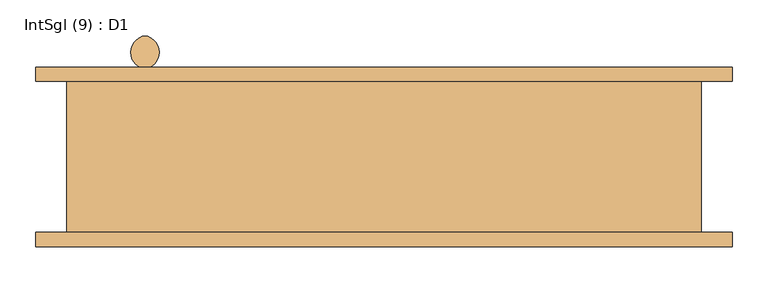
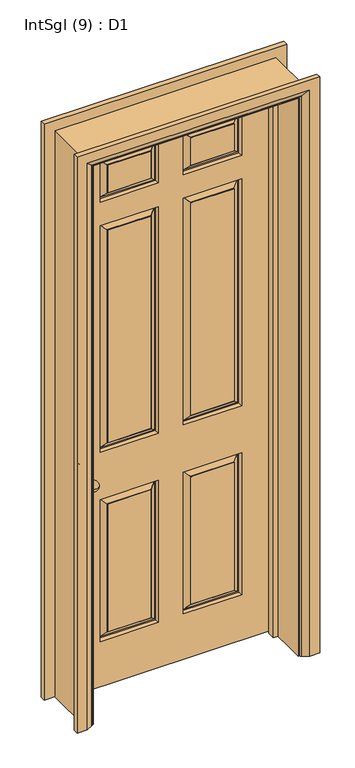
"""IFC4 building model written with IfcOpenShell, lengths in millimetres: door geometry, IntSgl (9) : D1."""

from ifc_helpers import new_model, si_unit, point, frame, origin, place, context, project, spatial, polyline, circle_curve, ellipse_curve, trimmed, outline, extrude, faceted_brep, source, transform, mapped, element, save
from ifc_brep_helpers import plane_surface, cylinder_surface, revolved_surface, advanced_brep


def intsgl_9_d1_fdab3a6c(model_context):
    return source(origin(), model_context, "Body", "SolidModel", [
        advanced_brep(
        [(-328.0, 48.0, 900.0), (-333.0, 3.562589, 900.0), (-338.0, 48.0, 900.0), (-338.0, 63.0, 900.0), (-328.0, 63.0, 900.0), (-353.0, 67.0, 900.0), (-313.0, 67.0, 900.0), (-353.0, 63.0, 900.0), (-313.0, 63.0, 900.0)],
        [
            (0, 1, circle_curve(frame((-336.1884862, 26.4213505, 900.0), z_axis=(0.0, 0.0, -1.0), x_axis=(0.0, 1.0, 0.0)), 23.0800654)),
            (1, 2, circle_curve(frame((-329.8115138, 26.4213505, 900.0), z_axis=(0.0, 0.0, -1.0), x_axis=(0.0, 1.0, 0.0)), 23.0800654)),
            (2, 0, circle_curve(frame((-333.0, 48.0, 900.0), z_axis=(0.0, -1.0, 0.0), x_axis=(-1.0, 0.0, 0.0)), 5.0)),
            (0, 2, circle_curve(frame((-333.0, 48.0, 900.0), z_axis=(0.0, -1.0, 0.0), x_axis=(-1.0, 0.0, 0.0)), 5.0)),
            (2, 3),
            (3, 4, circle_curve(frame((-333.0, 63.0, 900.0), z_axis=(0.0, -1.0, 0.0), x_axis=(-1.0, 0.0, 0.0)), 5.0)),
            (4, 0),
            (4, 3, circle_curve(frame((-333.0, 63.0, 900.0), z_axis=(0.0, -1.0, 0.0), x_axis=(-1.0, 0.0, 0.0)), 5.0)),
            (5, 6, circle_curve(frame((-333.0, 67.0, 900.0), z_axis=(0.0, 1.0, 0.0), x_axis=(1.0, 0.0, 0.0)), 20.0)),
            (6, 5, circle_curve(frame((-333.0, 67.0, 900.0), z_axis=(0.0, 1.0, 0.0), x_axis=(1.0, 0.0, 0.0)), 20.0)),
            (7, 8, circle_curve(frame((-333.0, 63.0, 900.0), z_axis=(0.0, -1.0, 0.0), x_axis=(1.0, 0.0, 0.0)), 20.0)),
            (8, 7, circle_curve(frame((-333.0, 63.0, 900.0), z_axis=(0.0, -1.0, 0.0), x_axis=(1.0, 0.0, 0.0)), 20.0)),
            (6, 8),
            (7, 5),
        ],
        [
            revolved_surface(trimmed(ellipse_curve(frame((-329.8115138, 26.4213505, 900.0), z_axis=(0.0, 0.0, -1.0), x_axis=(0.0, 1.0, 0.0)), 23.0800654, 23.0800654), [point((-333.0, 3.562589, 900.0))], [point((-338.0, 48.0, 900.0))], True, "CARTESIAN"), (-333.0, 63.0, 900.0), (0.0, 1.0, 0.0)),
            cylinder_surface(frame((-333.0, 63.0, 900.0), z_axis=(0.0, 1.0, 0.0), x_axis=(-1.0, 0.0, 0.0)), 5.0),
            plane_surface(frame((-313.0, 67.0, 900.0), z_axis=(0.0, 1.0, 0.0), x_axis=(0.0, 0.0, 1.0))),
            plane_surface(frame((-313.0, 63.0, 900.0), z_axis=(0.0, -1.0, 0.0), x_axis=(0.0, 0.0, -1.0))),
            cylinder_surface(frame((-333.0, 63.0, 900.0), z_axis=(0.0, 1.0, 0.0), x_axis=(1.0, 0.0, 0.0)), 20.0),
        ],
        [
            (0, [[1, 2, 3]]),
            (0, [[-1, 4, -2]]),
            (1, [[5, 6, 7, -3]]),
            (1, [[-7, 8, -5, -4]]),
            (2, [[9, 10]]),
            (3, [[11, 12], [-8, -6]]),
            (4, [[13, -11, 14, -10]]),
            (4, [[-14, -12, -13, -9]]),
        ],
    ),
        advanced_brep(
        [(-328.0, 124.0, 900.0), (-338.0, 124.0, 900.0), (-333.0, 168.437411, 900.0), (-328.0, 109.0, 900.0), (-338.0, 109.0, 900.0), (-353.0, 105.0, 900.0), (-313.0, 105.0, 900.0), (-353.0, 109.0, 900.0), (-313.0, 109.0, 900.0)],
        [
            (0, 1, circle_curve(frame((-333.0, 124.0, 900.0), z_axis=(0.0, 1.0, 0.0), x_axis=(-1.0, 0.0, 0.0)), 5.0)),
            (1, 2, circle_curve(frame((-329.8115138, 145.5786495, 900.0), z_axis=(0.0, 0.0, -1.0), x_axis=(0.0, -1.0, 0.0)), 23.0800654)),
            (2, 0, circle_curve(frame((-336.1884862, 145.5786495, 900.0), z_axis=(0.0, 0.0, -1.0), x_axis=(0.0, -1.0, 0.0)), 23.0800654)),
            (1, 0, circle_curve(frame((-333.0, 124.0, 900.0), z_axis=(0.0, 1.0, 0.0), x_axis=(-1.0, 0.0, 0.0)), 5.0)),
            (0, 3),
            (3, 4, circle_curve(frame((-333.0, 109.0, 900.0), z_axis=(0.0, 1.0, 0.0), x_axis=(-1.0, 0.0, 0.0)), 5.0)),
            (4, 1),
            (4, 3, circle_curve(frame((-333.0, 109.0, 900.0), z_axis=(0.0, 1.0, 0.0), x_axis=(-1.0, 0.0, 0.0)), 5.0)),
            (5, 6, circle_curve(frame((-333.0, 105.0, 900.0), z_axis=(0.0, -1.0, 0.0), x_axis=(1.0, 0.0, 0.0)), 20.0)),
            (6, 5, circle_curve(frame((-333.0, 105.0, 900.0), z_axis=(0.0, -1.0, 0.0), x_axis=(1.0, 0.0, 0.0)), 20.0)),
            (7, 8, circle_curve(frame((-333.0, 109.0, 900.0), z_axis=(0.0, 1.0, 0.0), x_axis=(1.0, 0.0, 0.0)), 20.0)),
            (8, 7, circle_curve(frame((-333.0, 109.0, 900.0), z_axis=(0.0, 1.0, 0.0), x_axis=(1.0, 0.0, 0.0)), 20.0)),
            (5, 7),
            (8, 6),
        ],
        [
            revolved_surface(trimmed(ellipse_curve(frame((-329.8115138, 145.5786495, 900.0), z_axis=(0.0, 0.0, 1.0), x_axis=(0.0, -1.0, 0.0)), 23.0800654, 23.0800654), [point((-333.0, 168.437411, 900.0))], [point((-338.0, 124.0, 900.0))], True, "CARTESIAN"), (-333.0, 109.0, 900.0), (0.0, -1.0, 0.0)),
            cylinder_surface(frame((-333.0, 109.0, 900.0), z_axis=(0.0, -1.0, 0.0), x_axis=(-1.0, 0.0, 0.0)), 5.0),
            plane_surface(frame((-313.0, 105.0, 900.0), z_axis=(0.0, -1.0, 0.0), x_axis=(0.0, 0.0, 1.0))),
            plane_surface(frame((-313.0, 109.0, 900.0), z_axis=(0.0, 1.0, 0.0), x_axis=(0.0, 0.0, -1.0))),
            cylinder_surface(frame((-333.0, 109.0, 900.0), z_axis=(0.0, -1.0, 0.0), x_axis=(1.0, 0.0, 0.0)), 20.0),
        ],
        [
            (0, [[1, 2, 3]]),
            (0, [[-2, 4, -3]]),
            (1, [[-1, 5, 6, 7]]),
            (1, [[-4, -7, 8, -5]]),
            (2, [[9, 10]]),
            (3, [[11, 12], [-6, -8]]),
            (4, [[-9, 13, -12, 14]]),
            (4, [[-10, -14, -11, -13]]),
        ],
    ),
        faceted_brep([(-408.0, 67.0, 2358.0), (-408.0, 67.0, 8.0), (408.0, 67.0, 8.0), (408.0, 67.0, 2358.0), (-50.0, 67.0, 800.0), (-50.0, 67.0, 200.0), (-283.0, 67.0, 200.0), (-283.0, 67.0, 800.0), (283.0, 67.0, 800.0), (283.0, 67.0, 200.0), (50.0, 67.0, 200.0), (50.0, 67.0, 800.0), (-50.0, 67.0, 1958.0), (-50.0, 67.0, 1000.0), (-283.0, 67.0, 1000.0), (-283.0, 67.0, 1958.0), (283.0, 67.0, 1958.0), (283.0, 67.0, 1000.0), (50.0, 67.0, 1000.0), (50.0, 67.0, 1958.0), (-50.0, 67.0, 2233.0), (-50.0, 67.0, 2058.0), (-283.0, 67.0, 2058.0), (-283.0, 67.0, 2233.0), (283.0, 67.0, 2233.0), (283.0, 67.0, 2058.0), (50.0, 67.0, 2058.0), (50.0, 67.0, 2233.0), (-80.0, 67.0, 230.0), (-80.0, 67.0, 770.0), (-253.0, 67.0, 770.0), (-253.0, 67.0, 230.0), (253.0, 67.0, 230.0), (253.0, 67.0, 770.0), (80.0, 67.0, 770.0), (80.0, 67.0, 230.0), (-80.0, 67.0, 1030.0), (-80.0, 67.0, 1928.0), (-253.0, 67.0, 1928.0), (-253.0, 67.0, 1030.0), (253.0, 67.0, 1030.0), (253.0, 67.0, 1928.0), (80.0, 67.0, 1928.0), (80.0, 67.0, 1030.0), (-80.0, 67.0, 2088.0), (-80.0, 67.0, 2203.0), (-253.0, 67.0, 2203.0), (-253.0, 67.0, 2088.0), (253.0, 67.0, 2088.0), (253.0, 67.0, 2203.0), (80.0, 67.0, 2203.0), (80.0, 67.0, 2088.0), (-408.0, 105.0, 2358.0), (408.0, 105.0, 2358.0), (408.0, 105.0, 8.0), (-408.0, 105.0, 8.0), (50.0, 105.0, 800.0), (50.0, 105.0, 200.0), (283.0, 105.0, 200.0), (283.0, 105.0, 800.0), (-283.0, 105.0, 800.0), (-283.0, 105.0, 200.0), (-50.0, 105.0, 200.0), (-50.0, 105.0, 800.0), (50.0, 105.0, 1958.0), (50.0, 105.0, 1000.0), (283.0, 105.0, 1000.0), (283.0, 105.0, 1958.0), (-283.0, 105.0, 1958.0), (-283.0, 105.0, 1000.0), (-50.0, 105.0, 1000.0), (-50.0, 105.0, 1958.0), (50.0, 105.0, 2233.0), (50.0, 105.0, 2058.0), (283.0, 105.0, 2058.0), (283.0, 105.0, 2233.0), (-283.0, 105.0, 2233.0), (-283.0, 105.0, 2058.0), (-50.0, 105.0, 2058.0), (-50.0, 105.0, 2233.0), (80.0, 105.0, 230.0), (80.0, 105.0, 770.0), (253.0, 105.0, 770.0), (253.0, 105.0, 230.0), (-253.0, 105.0, 230.0), (-253.0, 105.0, 770.0), (-80.0, 105.0, 770.0), (-80.0, 105.0, 230.0), (80.0, 105.0, 1030.0), (80.0, 105.0, 1928.0), (253.0, 105.0, 1928.0), (253.0, 105.0, 1030.0), (-253.0, 105.0, 1030.0), (-253.0, 105.0, 1928.0), (-80.0, 105.0, 1928.0), (-80.0, 105.0, 1030.0), (80.0, 105.0, 2088.0), (80.0, 105.0, 2203.0), (253.0, 105.0, 2203.0), (253.0, 105.0, 2088.0), (-253.0, 105.0, 2088.0), (-253.0, 105.0, 2203.0), (-80.0, 105.0, 2203.0), (-80.0, 105.0, 2088.0), (80.0, 104.0, 230.0), (80.0, 104.0, 770.0), (58.0, 90.0, 208.0), (58.0, 90.0, 792.0), (78.0, 104.0, 772.0), (78.0, 104.0, 228.0), (53.0, 90.0, 797.0), (53.0, 90.0, 203.0), (253.0, 104.0, 770.0), (275.0, 90.0, 792.0), (255.0, 104.0, 772.0), (280.0, 90.0, 797.0), (253.0, 104.0, 230.0), (275.0, 90.0, 208.0), (255.0, 104.0, 228.0), (280.0, 90.0, 203.0), (-253.0, 104.0, 230.0), (-253.0, 104.0, 770.0), (-275.0, 90.0, 208.0), (-275.0, 90.0, 792.0), (-255.0, 104.0, 772.0), (-255.0, 104.0, 228.0), (-280.0, 90.0, 797.0), (-280.0, 90.0, 203.0), (-80.0, 104.0, 770.0), (-58.0, 90.0, 792.0), (-78.0, 104.0, 772.0), (-53.0, 90.0, 797.0), (-80.0, 104.0, 230.0), (-58.0, 90.0, 208.0), (-78.0, 104.0, 228.0), (-53.0, 90.0, 203.0), (80.0, 104.0, 1030.0), (80.0, 104.0, 1928.0), (58.0, 90.0, 1008.0), (58.0, 90.0, 1950.0), (78.0, 104.0, 1930.0), (78.0, 104.0, 1028.0), (53.0, 90.0, 1955.0), (53.0, 90.0, 1003.0), (253.0, 104.0, 1928.0), (275.0, 90.0, 1950.0), (255.0, 104.0, 1930.0), (280.0, 90.0, 1955.0), (253.0, 104.0, 1030.0), (275.0, 90.0, 1008.0), (255.0, 104.0, 1028.0), (280.0, 90.0, 1003.0), (-253.0, 104.0, 1030.0), (-253.0, 104.0, 1928.0), (-275.0, 90.0, 1008.0), (-275.0, 90.0, 1950.0), (-255.0, 104.0, 1930.0), (-255.0, 104.0, 1028.0), (-280.0, 90.0, 1955.0), (-280.0, 90.0, 1003.0), (-80.0, 104.0, 1928.0), (-58.0, 90.0, 1950.0), (-78.0, 104.0, 1930.0), (-53.0, 90.0, 1955.0), (-80.0, 104.0, 1030.0), (-58.0, 90.0, 1008.0), (-78.0, 104.0, 1028.0), (-53.0, 90.0, 1003.0), (80.0, 104.0, 2088.0), (80.0, 104.0, 2203.0), (58.0, 90.0, 2066.0), (58.0, 90.0, 2225.0), (78.0, 104.0, 2205.0), (78.0, 104.0, 2086.0), (53.0, 90.0, 2230.0), (53.0, 90.0, 2061.0), (253.0, 104.0, 2203.0), (275.0, 90.0, 2225.0), (255.0, 104.0, 2205.0), (280.0, 90.0, 2230.0), (253.0, 104.0, 2088.0), (275.0, 90.0, 2066.0), (255.0, 104.0, 2086.0), (280.0, 90.0, 2061.0), (-253.0, 104.0, 2088.0), (-253.0, 104.0, 2203.0), (-275.0, 90.0, 2066.0), (-275.0, 90.0, 2225.0), (-255.0, 104.0, 2205.0), (-255.0, 104.0, 2086.0), (-280.0, 90.0, 2230.0), (-280.0, 90.0, 2061.0), (-80.0, 104.0, 2203.0), (-58.0, 90.0, 2225.0), (-78.0, 104.0, 2205.0), (-53.0, 90.0, 2230.0), (-80.0, 104.0, 2088.0), (-58.0, 90.0, 2066.0), (-78.0, 104.0, 2086.0), (-53.0, 90.0, 2061.0), (-80.0, 68.0, 230.0), (-80.0, 68.0, 770.0), (-58.0, 82.0, 208.0), (-58.0, 82.0, 792.0), (-78.0, 68.0, 772.0), (-78.0, 68.0, 228.0), (-53.0, 82.0, 797.0), (-53.0, 82.0, 203.0), (-253.0, 68.0, 770.0), (-275.0, 82.0, 792.0), (-255.0, 68.0, 772.0), (-280.0, 82.0, 797.0), (-253.0, 68.0, 230.0), (-275.0, 82.0, 208.0), (-255.0, 68.0, 228.0), (-280.0, 82.0, 203.0), (253.0, 68.0, 230.0), (253.0, 68.0, 770.0), (275.0, 82.0, 208.0), (275.0, 82.0, 792.0), (255.0, 68.0, 772.0), (255.0, 68.0, 228.0), (280.0, 82.0, 797.0), (280.0, 82.0, 203.0), (80.0, 68.0, 770.0), (58.0, 82.0, 792.0), (78.0, 68.0, 772.0), (53.0, 82.0, 797.0), (80.0, 68.0, 230.0), (58.0, 82.0, 208.0), (78.0, 68.0, 228.0), (53.0, 82.0, 203.0), (-80.0, 68.0, 1030.0), (-80.0, 68.0, 1928.0), (-58.0, 82.0, 1008.0), (-58.0, 82.0, 1950.0), (-78.0, 68.0, 1930.0), (-78.0, 68.0, 1028.0), (-53.0, 82.0, 1955.0), (-53.0, 82.0, 1003.0), (-253.0, 68.0, 1928.0), (-275.0, 82.0, 1950.0), (-255.0, 68.0, 1930.0), (-280.0, 82.0, 1955.0), (-253.0, 68.0, 1030.0), (-275.0, 82.0, 1008.0), (-255.0, 68.0, 1028.0), (-280.0, 82.0, 1003.0), (253.0, 68.0, 1030.0), (253.0, 68.0, 1928.0), (275.0, 82.0, 1008.0), (275.0, 82.0, 1950.0), (255.0, 68.0, 1930.0), (255.0, 68.0, 1028.0), (280.0, 82.0, 1955.0), (280.0, 82.0, 1003.0), (80.0, 68.0, 1928.0), (58.0, 82.0, 1950.0), (78.0, 68.0, 1930.0), (53.0, 82.0, 1955.0), (80.0, 68.0, 1030.0), (58.0, 82.0, 1008.0), (78.0, 68.0, 1028.0), (53.0, 82.0, 1003.0), (-80.0, 68.0, 2088.0), (-80.0, 68.0, 2203.0), (-58.0, 82.0, 2066.0), (-58.0, 82.0, 2225.0), (-78.0, 68.0, 2205.0), (-78.0, 68.0, 2086.0), (-53.0, 82.0, 2230.0), (-53.0, 82.0, 2061.0), (-253.0, 68.0, 2203.0), (-275.0, 82.0, 2225.0), (-255.0, 68.0, 2205.0), (-280.0, 82.0, 2230.0), (-253.0, 68.0, 2088.0), (-275.0, 82.0, 2066.0), (-255.0, 68.0, 2086.0), (-280.0, 82.0, 2061.0), (253.0, 68.0, 2088.0), (253.0, 68.0, 2203.0), (275.0, 82.0, 2066.0), (275.0, 82.0, 2225.0), (255.0, 68.0, 2205.0), (255.0, 68.0, 2086.0), (280.0, 82.0, 2230.0), (280.0, 82.0, 2061.0), (80.0, 68.0, 2203.0), (58.0, 82.0, 2225.0), (78.0, 68.0, 2205.0), (53.0, 82.0, 2230.0), (80.0, 68.0, 2088.0), (58.0, 82.0, 2066.0), (78.0, 68.0, 2086.0), (53.0, 82.0, 2061.0)], [[[0, 1, 2, 3], [4, 5, 6, 7], [8, 9, 10, 11], [12, 13, 14, 15], [16, 17, 18, 19], [20, 21, 22, 23], [24, 25, 26, 27]], [[28, 29, 30, 31]], [[32, 33, 34, 35]], [[36, 37, 38, 39]], [[40, 41, 42, 43]], [[44, 45, 46, 47]], [[48, 49, 50, 51]], [[52, 53, 54, 55], [56, 57, 58, 59], [60, 61, 62, 63], [64, 65, 66, 67], [68, 69, 70, 71], [72, 73, 74, 75], [76, 77, 78, 79]], [[80, 81, 82, 83]], [[84, 85, 86, 87]], [[88, 89, 90, 91]], [[92, 93, 94, 95]], [[96, 97, 98, 99]], [[100, 101, 102, 103]], [[1, 0, 52, 55]], [[2, 1, 55, 54]], [[3, 2, 54, 53]], [[0, 3, 53, 52]], [[104, 105, 81, 80]], [[106, 107, 108, 109]], [[56, 110, 111, 57]], [[81, 105, 112, 82]], [[108, 107, 113, 114]], [[110, 56, 59, 115]], [[82, 112, 116, 83]], [[114, 113, 117, 118]], [[115, 59, 58, 119]], [[104, 80, 83, 116]], [[109, 108, 114, 118], [105, 104, 116, 112]], [[106, 109, 118, 117]], [[111, 110, 115, 119], [107, 106, 117, 113]], [[57, 111, 119, 58]], [[120, 121, 85, 84]], [[122, 123, 124, 125]], [[60, 126, 127, 61]], [[85, 121, 128, 86]], [[124, 123, 129, 130]], [[126, 60, 63, 131]], [[86, 128, 132, 87]], [[130, 129, 133, 134]], [[131, 63, 62, 135]], [[120, 84, 87, 132]], [[125, 124, 130, 134], [121, 120, 132, 128]], [[122, 125, 134, 133]], [[127, 126, 131, 135], [123, 122, 133, 129]], [[61, 127, 135, 62]], [[136, 137, 89, 88]], [[138, 139, 140, 141]], [[64, 142, 143, 65]], [[89, 137, 144, 90]], [[140, 139, 145, 146]], [[142, 64, 67, 147]], [[90, 144, 148, 91]], [[146, 145, 149, 150]], [[147, 67, 66, 151]], [[136, 88, 91, 148]], [[141, 140, 146, 150], [137, 136, 148, 144]], [[138, 141, 150, 149]], [[143, 142, 147, 151], [139, 138, 149, 145]], [[65, 143, 151, 66]], [[152, 153, 93, 92]], [[154, 155, 156, 157]], [[68, 158, 159, 69]], [[93, 153, 160, 94]], [[156, 155, 161, 162]], [[158, 68, 71, 163]], [[94, 160, 164, 95]], [[162, 161, 165, 166]], [[163, 71, 70, 167]], [[152, 92, 95, 164]], [[157, 156, 162, 166], [153, 152, 164, 160]], [[154, 157, 166, 165]], [[159, 158, 163, 167], [155, 154, 165, 161]], [[69, 159, 167, 70]], [[168, 169, 97, 96]], [[170, 171, 172, 173]], [[72, 174, 175, 73]], [[97, 169, 176, 98]], [[172, 171, 177, 178]], [[174, 72, 75, 179]], [[98, 176, 180, 99]], [[178, 177, 181, 182]], [[179, 75, 74, 183]], [[168, 96, 99, 180]], [[173, 172, 178, 182], [169, 168, 180, 176]], [[170, 173, 182, 181]], [[175, 174, 179, 183], [171, 170, 181, 177]], [[73, 175, 183, 74]], [[184, 185, 101, 100]], [[186, 187, 188, 189]], [[76, 190, 191, 77]], [[101, 185, 192, 102]], [[188, 187, 193, 194]], [[190, 76, 79, 195]], [[102, 192, 196, 103]], [[194, 193, 197, 198]], [[195, 79, 78, 199]], [[184, 100, 103, 196]], [[189, 188, 194, 198], [185, 184, 196, 192]], [[186, 189, 198, 197]], [[191, 190, 195, 199], [187, 186, 197, 193]], [[77, 191, 199, 78]], [[200, 201, 29, 28]], [[202, 203, 204, 205]], [[4, 206, 207, 5]], [[29, 201, 208, 30]], [[204, 203, 209, 210]], [[206, 4, 7, 211]], [[30, 208, 212, 31]], [[210, 209, 213, 214]], [[211, 7, 6, 215]], [[200, 28, 31, 212]], [[205, 204, 210, 214], [201, 200, 212, 208]], [[202, 205, 214, 213]], [[207, 206, 211, 215], [203, 202, 213, 209]], [[5, 207, 215, 6]], [[216, 217, 33, 32]], [[218, 219, 220, 221]], [[8, 222, 223, 9]], [[33, 217, 224, 34]], [[220, 219, 225, 226]], [[222, 8, 11, 227]], [[34, 224, 228, 35]], [[226, 225, 229, 230]], [[227, 11, 10, 231]], [[216, 32, 35, 228]], [[221, 220, 226, 230], [217, 216, 228, 224]], [[218, 221, 230, 229]], [[223, 222, 227, 231], [219, 218, 229, 225]], [[9, 223, 231, 10]], [[232, 233, 37, 36]], [[234, 235, 236, 237]], [[12, 238, 239, 13]], [[37, 233, 240, 38]], [[236, 235, 241, 242]], [[238, 12, 15, 243]], [[38, 240, 244, 39]], [[242, 241, 245, 246]], [[243, 15, 14, 247]], [[232, 36, 39, 244]], [[237, 236, 242, 246], [233, 232, 244, 240]], [[234, 237, 246, 245]], [[239, 238, 243, 247], [235, 234, 245, 241]], [[13, 239, 247, 14]], [[248, 249, 41, 40]], [[250, 251, 252, 253]], [[16, 254, 255, 17]], [[41, 249, 256, 42]], [[252, 251, 257, 258]], [[254, 16, 19, 259]], [[42, 256, 260, 43]], [[258, 257, 261, 262]], [[259, 19, 18, 263]], [[248, 40, 43, 260]], [[253, 252, 258, 262], [249, 248, 260, 256]], [[250, 253, 262, 261]], [[255, 254, 259, 263], [251, 250, 261, 257]], [[17, 255, 263, 18]], [[264, 265, 45, 44]], [[266, 267, 268, 269]], [[20, 270, 271, 21]], [[45, 265, 272, 46]], [[268, 267, 273, 274]], [[270, 20, 23, 275]], [[46, 272, 276, 47]], [[274, 273, 277, 278]], [[275, 23, 22, 279]], [[264, 44, 47, 276]], [[269, 268, 274, 278], [265, 264, 276, 272]], [[266, 269, 278, 277]], [[271, 270, 275, 279], [267, 266, 277, 273]], [[21, 271, 279, 22]], [[280, 281, 49, 48]], [[282, 283, 284, 285]], [[24, 286, 287, 25]], [[49, 281, 288, 50]], [[284, 283, 289, 290]], [[286, 24, 27, 291]], [[50, 288, 292, 51]], [[290, 289, 293, 294]], [[291, 27, 26, 295]], [[280, 48, 51, 292]], [[285, 284, 290, 294], [281, 280, 292, 288]], [[282, 285, 294, 293]], [[287, 286, 291, 295], [283, 282, 293, 289]], [[25, 287, 295, 26]]]),
        faceted_brep([(-410.0, 105.0, 0.0), (-410.0, -105.0, 0.0), (-442.0, -105.0, 0.0), (-442.0, 105.0, 0.0), (-410.0, 105.0, 2360.0), (-410.0, -105.0, 2360.0), (-442.0, -105.0, 2392.0), (-442.0, 105.0, 2392.0), (410.0, 105.0, 0.0), (442.0, 105.0, 0.0), (442.0, -105.0, 0.0), (410.0, -105.0, 0.0), (410.0, 105.0, 2360.0), (442.0, 105.0, 2392.0), (442.0, -105.0, 2392.0), (410.0, -105.0, 2360.0)], [[[0, 1, 2, 3]], [[1, 0, 4, 5]], [[2, 1, 5, 6]], [[3, 2, 6, 7]], [[0, 3, 7, 4]], [[8, 9, 10, 11]], [[12, 13, 9, 8]], [[13, 14, 10, 9]], [[14, 15, 11, 10]], [[15, 12, 8, 11]], [[5, 4, 12, 15]], [[6, 5, 15, 14]], [[7, 6, 14, 13]], [[4, 7, 13, 12]]]),
        extrude(outline(polyline([(0.0, -410.0), (0.0, -391.0), (2341.0, -391.0), (2341.0, 391.0), (0.0, 391.0), (0.0, 410.0), (2360.0, 410.0), (2360.0, -410.0), (0.0, -410.0)])), frame((0.0, 33.0, 0.0), z_axis=(0.0, 1.0, 0.0), x_axis=(0.0, 0.0, 1.0)), (0.0, 0.0, 1.0), 32.0),
        advanced_brep(
        [(-485.0, -125.0, 0.0), (-485.0, -105.0, 0.0), (-415.0, -105.0, 0.0), (-419.0, -111.0, 0.0), (-445.0, -125.0, 0.0), (-485.0, -125.0, 2435.0), (-485.0, -105.0, 2435.0), (485.0, -105.0, 2435.0), (485.0, -105.0, 0.0), (415.0, -105.0, 0.0), (415.0, -105.0, 2365.0), (-415.0, -105.0, 2365.0), (-419.0, -111.0, 2369.0), (-445.0, -125.0, 2395.0), (445.0, -125.0, 2395.0), (445.0, -125.0, 0.0), (485.0, -125.0, 0.0), (485.0, -125.0, 2435.0), (419.0, -111.0, 0.0), (419.0, -111.0, 2369.0)],
        [
            (0, 1),
            (1, 2),
            (2, 3, circle_curve(frame((-423.0, -104.0, 0.0), z_axis=(0.0, 0.0, -1.0), x_axis=(-1.0, 0.0, 0.0)), 8.0622577)),
            (3, 4),
            (4, 0),
            (0, 5),
            (5, 6),
            (6, 1),
            (6, 7),
            (7, 8),
            (8, 9),
            (9, 10),
            (10, 11),
            (11, 2),
            (11, 12, ellipse_curve(frame((-423.0, -104.0, 2373.0), z_axis=(-0.7071067811865475, 0.0, -0.7071067811865475), x_axis=(0.7071067811865474, 0.0, -0.7071067811865476)), 11.4017543, 8.0622577)),
            (12, 3),
            (12, 13),
            (13, 4),
            (13, 14),
            (14, 15),
            (15, 16),
            (16, 17),
            (17, 5),
            (7, 17),
            (16, 8),
            (15, 18),
            (18, 9, circle_curve(frame((423.0, -104.0, 0.0), z_axis=(0.0, 0.0, -1.0), x_axis=(1.0, 0.0, 0.0)), 8.0622577)),
            (19, 10, ellipse_curve(frame((423.0, -104.0, 2373.0), z_axis=(0.7071067811865475, 0.0, -0.7071067811865475), x_axis=(0.7071067811865474, 0.0, 0.7071067811865476)), 11.4017543, 8.0622577)),
            (18, 19),
            (14, 19),
            (19, 12),
        ],
        [
            plane_surface(frame((-415.0, -105.0, 0.0), z_axis=(0.0, 0.0, -1.0), x_axis=(0.0, -1.0, 0.0))),
            plane_surface(frame((-485.0, -125.0, 0.0), z_axis=(-1.0, 0.0, 0.0), x_axis=(0.0, 0.0, 1.0))),
            plane_surface(frame((-485.0, -105.0, 0.0), z_axis=(0.0, 1.0, 0.0), x_axis=(0.0, 0.0, 1.0))),
            cylinder_surface(frame((-423.0, -104.0, 0.0), z_axis=(0.0, 0.0, -1.0), x_axis=(-1.0, 0.0, 0.0)), 8.0622577),
            plane_surface(frame((-419.0, -111.0, 0.0), z_axis=(0.4740998230350183, -0.8804710999221749, 0.0), x_axis=(0.0, 0.0, 1.0))),
            plane_surface(frame((-445.0, -125.0, 0.0), z_axis=(0.0, -1.0, 0.0), x_axis=(0.0, 0.0, 1.0))),
            plane_surface(frame((485.0, -125.0, 2435.0), z_axis=(1.0, 0.0, 0.0), x_axis=(0.0, 0.0, -1.0))),
            plane_surface(frame((415.0, -105.0, 0.0), z_axis=(0.0, 0.0, -1.0), x_axis=(0.0, -1.0, 0.0))),
            cylinder_surface(frame((423.0, -104.0, 2365.0), z_axis=(0.0, 0.0, 1.0), x_axis=(1.0, 0.0, 0.0)), 8.0622577),
            plane_surface(frame((419.0, -111.0, 2369.0), z_axis=(-0.4740998230350183, -0.8804710999221749, 0.0), x_axis=(0.0, 0.0, -1.0))),
            plane_surface(frame((-485.0, -125.0, 2435.0), z_axis=(0.0, 0.0, 1.0), x_axis=(1.0, 0.0, 0.0))),
            cylinder_surface(frame((-415.0, -104.0, 2373.0), z_axis=(-1.0, 0.0, 0.0), x_axis=(0.0, 0.0, 1.0)), 8.0622577),
            plane_surface(frame((-419.0, -111.0, 2369.0), z_axis=(0.0, -0.8804710999221749, -0.4740998230350183), x_axis=(1.0, 0.0, 0.0))),
        ],
        [
            (0, [[1, 2, 3, 4, 5]]),
            (1, [[-1, 6, 7, 8]]),
            (2, [[-2, -8, 9, 10, 11, 12, 13, 14]]),
            (3, [[-3, -14, 15, 16]]),
            (4, [[-4, -16, 17, 18]]),
            (5, [[-5, -18, 19, 20, 21, 22, 23, -6]]),
            (6, [[24, -22, 25, -10]]),
            (7, [[-21, 26, 27, -11, -25]]),
            (8, [[28, -12, -27, 29]]),
            (9, [[30, -29, -26, -20]]),
            (10, [[-7, -23, -24, -9]]),
            (11, [[-15, -13, -28, 31]]),
            (12, [[-17, -31, -30, -19]]),
        ],
    ),
        advanced_brep(
        [(485.0, 125.0, 0.0), (485.0, 105.0, 0.0), (415.0, 105.0, 0.0), (419.0, 111.0, 0.0), (445.0, 125.0, 0.0), (485.0, 125.0, 2435.0), (485.0, 105.0, 2435.0), (-485.0, 105.0, 2435.0), (-485.0, 105.0, 0.0), (-415.0, 105.0, 0.0), (-415.0, 105.0, 2365.0), (415.0, 105.0, 2365.0), (419.0, 111.0, 2369.0), (445.0, 125.0, 2395.0), (-445.0, 125.0, 2395.0), (-445.0, 125.0, 0.0), (-485.0, 125.0, 0.0), (-485.0, 125.0, 2435.0), (-419.0, 111.0, 0.0), (-419.0, 111.0, 2369.0)],
        [
            (0, 1),
            (1, 2),
            (2, 3, circle_curve(frame((423.0, 104.0, 0.0), z_axis=(0.0, 0.0, -1.0), x_axis=(1.0, 0.0, 0.0)), 8.0622577)),
            (3, 4),
            (4, 0),
            (0, 5),
            (5, 6),
            (6, 1),
            (6, 7),
            (7, 8),
            (8, 9),
            (9, 10),
            (10, 11),
            (11, 2),
            (11, 12, ellipse_curve(frame((423.0, 104.0, 2373.0), z_axis=(0.7071067811865475, 0.0, -0.7071067811865475), x_axis=(-0.7071067811865474, 0.0, -0.7071067811865476)), 11.4017543, 8.0622577)),
            (12, 3),
            (12, 13),
            (13, 4),
            (13, 14),
            (14, 15),
            (15, 16),
            (16, 17),
            (17, 5),
            (7, 17),
            (16, 8),
            (15, 18),
            (18, 9, circle_curve(frame((-423.0, 104.0, 0.0), z_axis=(0.0, 0.0, -1.0), x_axis=(-1.0, 0.0, 0.0)), 8.0622577)),
            (19, 10, ellipse_curve(frame((-423.0, 104.0, 2373.0), z_axis=(-0.7071067811865475, 0.0, -0.7071067811865475), x_axis=(-0.7071067811865474, 0.0, 0.7071067811865476)), 11.4017543, 8.0622577)),
            (18, 19),
            (14, 19),
            (19, 12),
        ],
        [
            plane_surface(frame((415.0, 105.0, 0.0), z_axis=(0.0, 0.0, -1.0), x_axis=(0.0, 1.0, 0.0))),
            plane_surface(frame((485.0, 125.0, 0.0), z_axis=(1.0, 0.0, 0.0), x_axis=(0.0, 0.0, 1.0))),
            plane_surface(frame((485.0, 105.0, 0.0), z_axis=(0.0, -1.0, 0.0), x_axis=(0.0, 0.0, 1.0))),
            cylinder_surface(frame((423.0, 104.0, 0.0), z_axis=(0.0, 0.0, -1.0), x_axis=(1.0, 0.0, 0.0)), 8.0622577),
            plane_surface(frame((419.0, 111.0, 0.0), z_axis=(-0.4740998230350183, 0.8804710999221749, 0.0), x_axis=(0.0, 0.0, 1.0))),
            plane_surface(frame((445.0, 125.0, 0.0), z_axis=(0.0, 1.0, 0.0), x_axis=(0.0, 0.0, 1.0))),
            plane_surface(frame((-485.0, 125.0, 2435.0), z_axis=(-1.0, 0.0, 0.0), x_axis=(0.0, 0.0, -1.0))),
            plane_surface(frame((-415.0, 105.0, 0.0), z_axis=(0.0, 0.0, -1.0), x_axis=(0.0, 1.0, 0.0))),
            cylinder_surface(frame((-423.0, 104.0, 2365.0), z_axis=(0.0, 0.0, 1.0), x_axis=(-1.0, 0.0, 0.0)), 8.0622577),
            plane_surface(frame((-419.0, 111.0, 2369.0), z_axis=(0.4740998230350183, 0.8804710999221749, 0.0), x_axis=(0.0, 0.0, -1.0))),
            plane_surface(frame((485.0, 125.0, 2435.0), z_axis=(0.0, 0.0, 1.0), x_axis=(-1.0, 0.0, 0.0))),
            cylinder_surface(frame((415.0, 104.0, 2373.0), z_axis=(1.0, 0.0, 0.0), x_axis=(0.0, 0.0, 1.0)), 8.0622577),
            plane_surface(frame((419.0, 111.0, 2369.0), z_axis=(0.0, 0.8804710999221749, -0.4740998230350183), x_axis=(-1.0, 0.0, 0.0))),
        ],
        [
            (0, [[1, 2, 3, 4, 5]]),
            (1, [[-1, 6, 7, 8]]),
            (2, [[-2, -8, 9, 10, 11, 12, 13, 14]]),
            (3, [[-3, -14, 15, 16]]),
            (4, [[-4, -16, 17, 18]]),
            (5, [[-5, -18, 19, 20, 21, 22, 23, -6]]),
            (6, [[24, -22, 25, -10]]),
            (7, [[-21, 26, 27, -11, -25]]),
            (8, [[28, -12, -27, 29]]),
            (9, [[30, -29, -26, -20]]),
            (10, [[-7, -23, -24, -9]]),
            (11, [[-15, -13, -28, 31]]),
            (12, [[-17, -31, -30, -19]]),
        ],
    ),
    ])


if __name__ == "__main__":
    model = new_model("IFC4")
    model_context = context("Model", 3, world=origin())
    ifc_project = project(units=[si_unit("LENGTHUNIT", "METRE", prefix="MILLI")], contexts=[model_context])
    site = spatial("IfcSite", under=ifc_project)
    building = spatial("IfcBuilding", under=site)
    placement = place(None, origin())
    intsgl_9_d1_shape = intsgl_9_d1_fdab3a6c(model_context)
    element("IfcDoor", 1, ObjectType="IntSgl (9) : D1", at=placement, inside=building, context=model_context, shape_type="MappedRepresentation", body=[
        mapped(intsgl_9_d1_shape, transform((0.0, 0.0, 0.0), x_axis=(1.0, 0.0, 0.0), y_axis=(0.0, 1.0, 0.0), z_axis=(0.0, 0.0, 1.0))),
    ])
    save(model, "model.ifc")

# Revit data of these elements
# Type "IntSgl (9) : D1"
#   Type Mark = "49"
#   Operation = "SingleSwingRight"
#   Manufacturer = "Revit"
#   Keynote = "L20"
#   UnderCut = 8 mm
#   Tolerance = 2 mm
#   Thickness = 38 mm
#   Structural Tolerance = 8 mm
#   StopDepth = 32 mm
#   Stop Thickness = 19 mm
#   Stile Top Rail = 125 mm
#   Stile Shutting = 125 mm
#   Stile Muntin Rail = 100 mm
#   Stile Lock Rail = 200 mm
#   Stile Intermediate/Frieze = 100 mm
#   Stile Hanging = 125 mm
#   Stile Bottom Rail = 200 mm
#   Rough Width = 900 mm
#   Rough Height = 2400 mm
#   Height to Top Lock Rail = 1000 mm
#   Handle Z Distance = 900 mm
#   Handle X Distance = 75 mm
#   Frame Thickness = 32 mm
#   Door Panel Width = 816 mm
#   Height = 2400 mm
#   Width = 900 mm
#   Door Panel Thickness = 38 mm
#   Door Panel Offset = 0 mm
#   Door Panel Height = 2350 mm
#   Architrave Setback = 5 mm
#   Vis - Ironmongery = yes
#   Material Ironmongery = Door - Handle
#   Material Frame = Door - Frame/Mullion
#   Material Door = Door - Panel
#   Material Architrave = Door - Architrave
#   Function = (empty or 0)
#   Wall Closure = (empty or 0)
# Element 1 (IfcDoor, "IntSgl (9) : D1")
#   Materials on its faces: "Door - Panel", "Door - Architrave", "Door - Frame/Mullion", "Door - Handle"
# Materials
#   "Door - Handle": colour RGB 0 0 0, transparency 0, Keynote = "P21", Cost = 0, Export to IFC = 0
#   "Door - Frame/Mullion": class "Wood", colour RGB 212 179 113, transparency 0, Keynote = "L20", Cost = 0, Export to IFC = 0
#   "Door - Panel": class "Wood", colour RGB 210 159 95, transparency 0, Keynote = "L20", Cost = 0, Export to IFC = 0
#   "Door - Architrave": class "Wood", colour RGB 154 90 5, transparency 0, Keynote = "P20", Cost = 0, Export to IFC = 0
